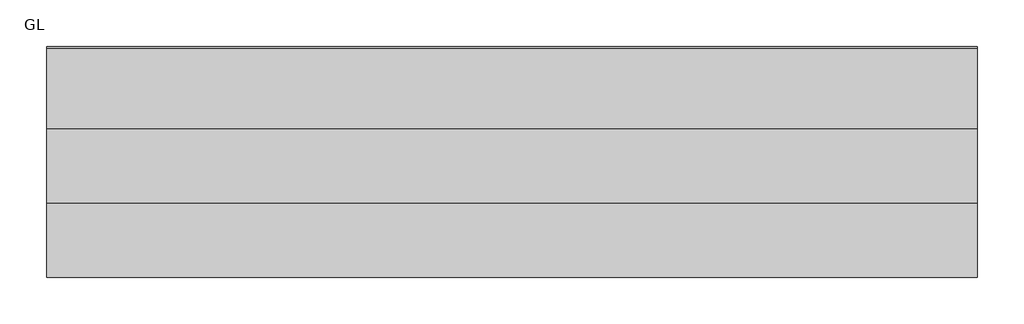
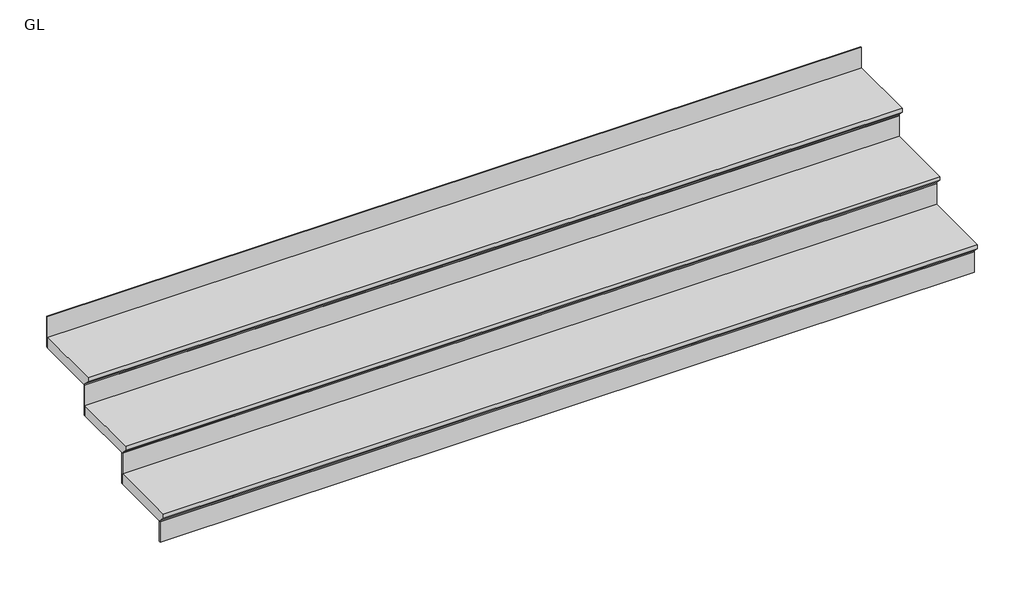
# One storey: 1 stair flight.
"""IFC4 building model written with IfcOpenShell, lengths in millimetres."""

from ifc_helpers import new_model, si_unit, origin, place, context, project, spatial, transform, mapped, element, save
from components import stair_flight_523d9302

model = new_model("IFC4")

# Units and contexts
model_context = context("Model", 3, world=origin())
ifc_project = project(units=[si_unit("LENGTHUNIT", "METRE", prefix="MILLI")], contexts=[model_context])

# Site, building, storey
site = spatial("IfcSite", under=ifc_project)
building = spatial("IfcBuilding", under=site)
storey = spatial("IfcBuildingStorey", under=building, Name="GL", Elevation=-609.6)

# Stair flight
placement = place(None, origin())
stair_flight_shape = stair_flight_523d9302(model_context)
element("IfcStairFlight", 1, ObjectType="2\" Tread 1\" Nosing 1/4\" Riser", at=placement, inside=storey, context=model_context, shape_type="MappedRepresentation", body=[
    mapped(stair_flight_shape, transform((0.0, 0.0, 0.0), x_axis=(1.0, 0.0, 0.0), y_axis=(0.0, 1.0, 0.0), z_axis=(0.0, 0.0, 1.0))),
])

save(model, "model.ifc")

# Revit data of these elements
# Element 1 (IfcStairFlight, "2\" Tread 1\" Nosing 1/4\" Riser")
#   Phase Created = New Construction
